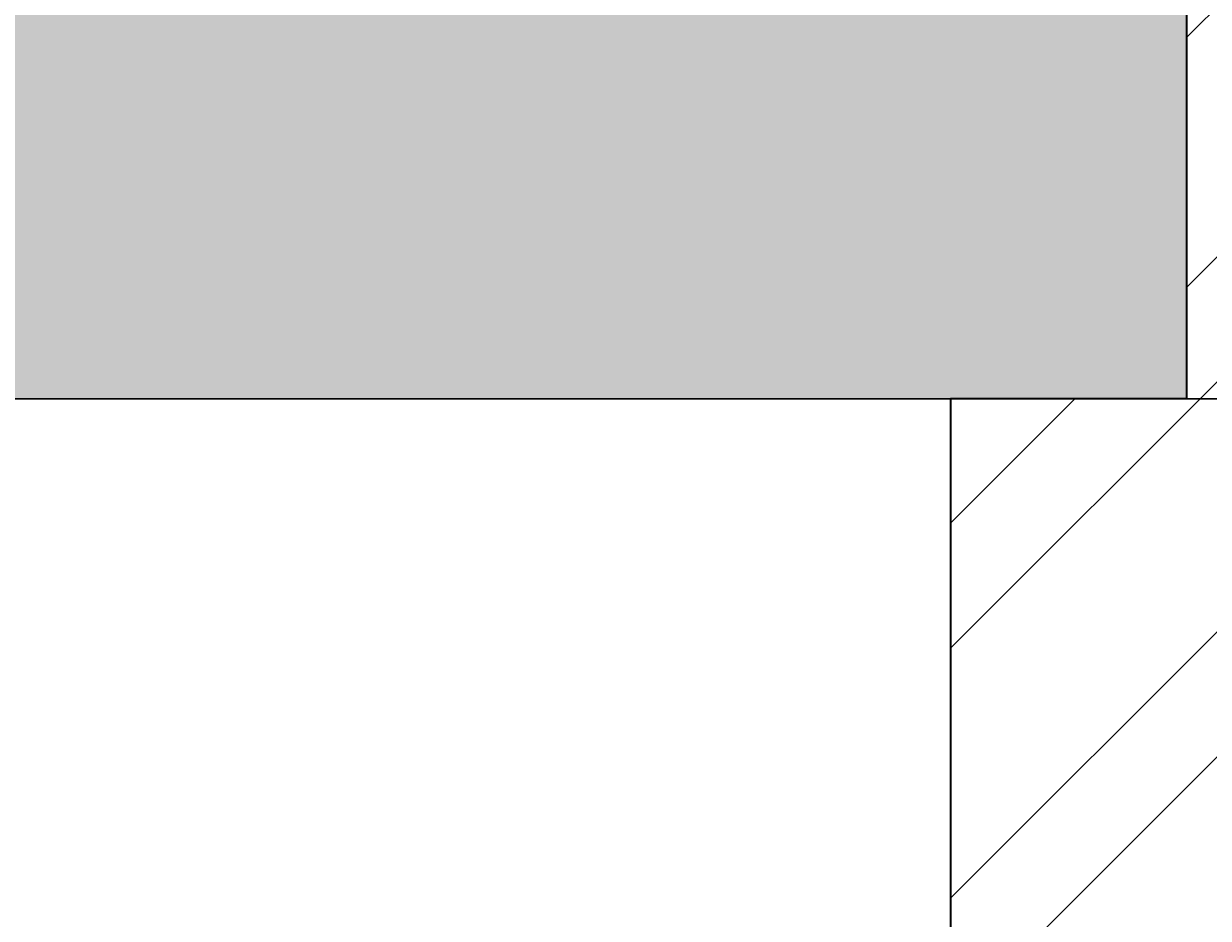
# Model space of a CAD drawing. Units: inches. Extents: x -301 to 715, y -607 to 364.
# Tile 8 of 141: x -66 to -41, y -492 to -474. Entities that reach past the tile are written whole.
import ezdxf

# ---------------------------------------------------------------- set-up
doc = ezdxf.new("R2010")
doc.units = ezdxf.units.IN
doc.header["$MEASUREMENT"] = 0
for name, color, linetype, lineweight in [('A-ANNO-DIMS', 2, 'Continuous', 18), ('A-GRND', 7, 'Continuous', 25), ('A-SECT', 1, 'Continuous', 35), ('A-SECT-PATT', 8, 'Continuous', 13), ('S-FNDN', 2, 'Continuous', 35)]:
    doc.layers.add(name, color=color, linetype=linetype, lineweight=lineweight)
doc.styles.get("Standard").update_dxf_attribs({"font": 'arial.ttf'})
doc.dimstyles.get("Standard").update_dxf_attribs({"dimtxt": 0.18, "dimasz": 0.18, "dimexe": 0.18, "dimexo": 0.0625, "dimgap": 0.09, "dimtad": 0, "dimtih": 1, "dimtoh": 1, "dimdec": 1, "dimzin": 0, "dimdsep": 46, "dimlunit": 4, "dimtxsty": 'Standard', "dimcen": 0.09, "dimclrd": 3, "dimclre": 4, "dimclrt": 6, "dimadec": 0, "dimazin": 0, "dimtfac": 1, "dimtdec": 1, "dimtofl": 0, "dimtmove": 0, "dimatfit": 3, "dimfxl": 1, "dimtfill": 2, "dimtfillclr": 51, "dimtolj": 1, "dimtzin": 0, "dimarcsym": 0})

# ---------------------------------------------------------------- blocks, each defined once
blk = doc.blocks.new('*D179')
at = {"layer": 'A-ANNO-DIMS', "color": 4, "lineweight": -2, "transparency": 16777216}
for p, q in [((-87.981, -433.54), (-87.981, -573.809)), ((-35.282, -463.54), (-35.282, -573.809))]:
    blk.add_line(p, q, dxfattribs=at)
at = {"layer": 'A-ANNO-DIMS', "color": 3, "lineweight": -2, "transparency": 16777216}
for p, q in [((-87.801, -573.629), (-62.174, -573.629)), ((-35.462, -573.629), (-61.089, -573.629))]:
    blk.add_line(p, q, dxfattribs=at)
at = {"layer": 'A-ANNO-DIMS', "color": 3, "transparency": 16777216}
for points in [[(-87.801, -573.599), (-87.801, -573.659), (-87.981, -573.629)], [(-35.462, -573.599), (-35.462, -573.659), (-35.282, -573.629)]]:
    blk.add_solid(points, dxfattribs=at)
at = {"layer": 'Defpoints', "color": 0, "transparency": 16777216}
for p in [(-87.981, -433.477), (-35.282, -463.477), (-35.282, -573.629)]:
    blk.add_point(p, dxfattribs=at)
at = {"layer": 'A-ANNO-DIMS', "color": 6, "transparency": 16777216, "insert": (-61.631, -573.629), "char_height": 0.18, "attachment_point": 5, "bg_fill": 1, "box_fill_scale": 1.25, "bg_fill_color": 51, "bg_fill_transparency": 0}
blk.add_mtext('\\A1;4\'-4 1/2"', dxfattribs=at)
blk = doc.blocks.new('*D190')
at = {"layer": 'A-ANNO-DIMS', "color": 4, "lineweight": -2, "transparency": 16777216}
for p, q in [((129.193, -481.477), (-266.112, -481.477)), ((124.193, -511.477), (-266.112, -511.477))]:
    blk.add_line(p, q, dxfattribs=at)
at = {"layer": 'A-ANNO-DIMS', "color": 3, "lineweight": -2, "transparency": 16777216}
for p, q in [((-265.932, -481.657), (-265.932, -496.296)), ((-265.932, -511.297), (-265.932, -496.659))]:
    blk.add_line(p, q, dxfattribs=at)
at = {"layer": 'A-ANNO-DIMS', "color": 3, "transparency": 16777216}
for points in [[(-265.962, -481.657), (-265.902, -481.657), (-265.932, -481.477)], [(-265.962, -511.297), (-265.902, -511.297), (-265.932, -511.477)]]:
    blk.add_solid(points, dxfattribs=at)
at = {"layer": 'Defpoints', "color": 0, "transparency": 16777216}
for p in [(129.255, -481.477), (-265.932, -511.477), (124.255, -511.477)]:
    blk.add_point(p, dxfattribs=at)
at = {"layer": 'A-ANNO-DIMS', "color": 6, "transparency": 16777216, "insert": (-265.932, -496.477), "char_height": 0.18, "attachment_point": 5, "bg_fill": 1, "box_fill_scale": 1.25, "bg_fill_color": 51, "bg_fill_transparency": 0}
blk.add_mtext('\\A1;2\'-6"', dxfattribs=at)
blk = doc.blocks.new('*D191')
at = {"layer": 'A-ANNO-DIMS', "color": 4, "lineweight": -2, "transparency": 16777216}
for p, q in [((129.193, -481.477), (-266.112, -481.477)), ((114.193, -540.477), (-266.112, -540.477))]:
    blk.add_line(p, q, dxfattribs=at)
at = {"layer": 'A-ANNO-DIMS', "color": 3, "lineweight": -2, "transparency": 16777216}
for p, q in [((-265.932, -481.657), (-265.932, -510.797)), ((-265.932, -540.297), (-265.932, -511.158))]:
    blk.add_line(p, q, dxfattribs=at)
at = {"layer": 'A-ANNO-DIMS', "color": 3, "transparency": 16777216}
for points in [[(-265.962, -481.657), (-265.902, -481.657), (-265.932, -481.477)], [(-265.962, -540.297), (-265.902, -540.297), (-265.932, -540.477)]]:
    blk.add_solid(points, dxfattribs=at)
at = {"layer": 'Defpoints', "color": 0, "transparency": 16777216}
for p in [(129.255, -481.477), (-265.932, -540.477), (114.255, -540.477)]:
    blk.add_point(p, dxfattribs=at)
at = {"layer": 'A-ANNO-DIMS', "color": 6, "transparency": 16777216, "insert": (-265.932, -510.977), "char_height": 0.18, "attachment_point": 5, "bg_fill": 1, "box_fill_scale": 1.25, "bg_fill_color": 51, "bg_fill_transparency": 0}
blk.add_mtext('\\A1;4\'-11"', dxfattribs=at)

msp = doc.modelspace()

# ---------------------------------------------------------------- hatches: boundary and pattern name
at = {"layer": 'A-SECT-PATT'}
h = msp.add_hatch(dxfattribs=at)
h.set_pattern_fill('ANSI32', color=256, scale=15)
h.set_pattern_definition([(45, (10.321, 33.8764), (-3.977476, 3.977476), []), (45, (12.973, 33.8764), (-3.977476, 3.977476), [])])
h.paths.add_polyline_path([(-185.282, -324.477), (-199.282, -324.477), (-199.282, -329.477), (-194.282, -329.477), (-194.282, -353.477), (-185.282, -353.477)])
h.paths.add_polyline_path([(-185.282, -361.477), (-193.904, -361.477), (-193.982, -377.537), (-185.282, -377.537)])
h.paths.add_polyline_path([(143.218, -329.477), (148.218, -329.477), (148.218, -324.477), (134.255, -324.477), (134.255, -353.477), (143.218, -353.477)])
h.paths.add_polyline_path([(143.218, -361.477), (134.255, -361.477), (134.255, -377.477), (143.218, -377.477)])
h.paths.add_polyline_path([(-185.282, -439.477), (-194.282, -439.477), (-194.282, -463.477), (-185.282, -463.477)])
h.paths.add_polyline_path([(-185.282, -471.477), (-194.282, -471.477), (-194.282, -481.477), (-185.282, -481.477)])
h.paths.add_polyline_path([(-185.282, -463.477), (-194.282, -463.477), (-194.282, -466.477), (-185.282, -466.477)])
h.paths.add_polyline_path([(-185.282, -466.477), (-194.282, -466.477), (-194.282, -471.477), (-185.282, -471.477)])
h.paths.add_polyline_path([(-180.282, -481.477), (-185.282, -481.477), (-194.282, -481.477), (-199.282, -481.477), (-199.282, -493.477), (-180.282, -493.477)])
h.paths.add_polyline_path([(-175.282, -493.477), (-180.282, -493.477), (-199.282, -493.477), (-204.282, -493.477), (-204.282, -511.477), (-175.282, -511.477)])
h.paths.add_polyline_path([(-170.282, -511.477), (-175.282, -511.477), (-204.282, -511.477), (-209.282, -511.477), (-209.282, -535.477), (-170.282, -535.477)])
h.paths.add_polyline_path([(-35.282, -463.477), (-41.282, -463.477), (-41.282, -466.477), (-35.282, -466.477)])
h.paths.add_polyline_path([(-35.282, -466.477), (-41.282, -466.477), (-41.282, -471.477), (-35.282, -471.477)])
h.paths.add_polyline_path([(-35.282, -471.477), (-41.282, -471.477), (-41.282, -481.477), (-35.282, -481.477)])
h.paths.add_polyline_path([(-30.282, -481.477), (-46.282, -481.477), (-46.282, -493.477), (-30.282, -493.477)])
h.paths.add_polyline_path([(-25.282, -493.477), (-30.282, -493.477), (-46.282, -493.477), (-51.282, -493.477), (-51.282, -511.477), (-25.282, -511.477)])
h.paths.add_polyline_path([(-20.282, -511.477), (-25.282, -511.477), (-51.282, -511.477), (-56.282, -511.477), (-56.282, -535.477), (-20.282, -535.477)])
h.paths.add_polyline_path([(143.218, -463.477), (134.255, -463.477), (134.255, -466.477), (143.218, -466.477)])
h.paths.add_polyline_path([(143.218, -466.477), (134.255, -466.477), (134.255, -471.477), (143.218, -471.477)])
h.paths.add_polyline_path([(143.218, -471.477), (134.255, -471.477), (134.255, -481.477), (143.218, -481.477)])
h.paths.add_polyline_path([(148.255, -481.477), (143.255, -481.477), (134.255, -481.477), (129.255, -481.477), (129.255, -493.477), (148.255, -493.477)])
h.paths.add_polyline_path([(153.255, -493.477), (148.255, -493.477), (129.255, -493.477), (124.255, -493.477), (124.255, -511.477), (153.255, -511.477)])
h.paths.add_polyline_path([(158.255, -511.477), (153.255, -511.477), (124.255, -511.477), (119.255, -511.477), (119.255, -535.477), (158.255, -535.477)])
h = msp.add_hatch(dxfattribs=at)
h.set_pattern_fill('AR-CONC', color=256, scale=0.5)
h.set_pattern_definition([(50, (10.3213, 33.8764), (3.586301, -0.31376), [0.375, -4.125]), (355, (10.3213, 33.8764), (-0.693757, 3.76096), [0.3, -3.3]), (100.45144, (10.62, 33.8502), (2.892544, 3.4472), [0.3187, -3.50571]), (46.1842, (10.3213, 34.8764), (5.336207, -0.827596), [0.5625, -6.1875]), (96.6356, (10.766, 34.8074), (4.67331, 4.870593), [0.47805, -5.25857]), (351.1842, (10.321, 34.8764), (4.67331, 4.870593), [0.45, -4.95]), (21, (10.8213, 34.6264), (2.984535, -2.013094), [0.375, -4.125]), (326, (10.8213, 34.6264), (1.216577, 3.62575), [0.3, -3.3]), (71.45144, (11.07, 34.4586), (4.201112, 1.612656), [0.3187, -3.50571]), (37.5, (10.3213, 33.8764), (0.0607993, 1.6644693), [0, -3.26, 0, -3.35, 0, -3.3125]), (7.5, (10.3213, 33.8764), (1.3153477, 1.9720586), [0, -1.91, 0, -3.185, 0, -1.2625]), (327.5, (9.2063, 33.8764), (2.6691122, -0.1127744), [0, -1.25, 0, -3.9, 0, -5.175]), (317.5, (8.7063, 33.8764), (2.915931, 0.500525), [0, -1.625, 0, -2.59, 0, -3.675])])
h.paths.add_polyline_path([(-56.282, -535.477), (-61.282, -535.477), (-61.282, -540.477), (-15.282, -540.477), (-15.282, -535.477), (-20.282, -535.477)])
h.paths.add_polyline_path([(119.255, -535.477), (114.255, -535.477), (114.255, -540.477), (163.255, -540.477), (163.255, -535.477), (158.255, -535.477)])
h.paths.add_polyline_path([(-206.282, -471.477), (-209.282, -471.477), (-209.282, -481.477), (-206.282, -481.477), (-194.282, -481.477), (-194.282, -471.477)])
h.paths.add_polyline_path([(-41.282, -481.477), (-41.282, -471.477), (-185.282, -471.477), (-185.282, -481.477), (-180.282, -481.477)])
h.paths.add_polyline_path([(134.255, -481.477), (134.255, -471.477), (-35.282, -471.477), (-35.282, -481.477), (-30.282, -481.477)])
h.paths.add_polyline_path([(155.218, -481.477), (158.218, -481.477), (158.218, -471.477), (153.218, -471.477), (143.218, -471.477), (143.218, -481.477), (148.255, -481.477)])
h.paths.add_polyline_path([(-193.88, -356.477), (-193.904, -361.477), (143.218, -361.477), (143.218, -356.477)])

# ---------------------------------------------------------------- linework, layer by layer
at = {"layer": 'A-GRND'}
msp.add_line((-206.282, -481.477), (155.218, -481.477), dxfattribs=at)
at = {"layer": 'A-SECT'}
msp.add_line((-41.282, -361.477), (-41.282, -481.477), dxfattribs=at)
at = {"layer": 'S-FNDN'}
for p, q in [((-41.282, -481.477), (-46.282, -481.477)), ((-46.282, -481.477), (-46.282, -493.477))]:
    msp.add_line(p, q, dxfattribs=at)

# ---------------------------------------------------------------- dimensions: what is measured, and where the dimension line sits
at = {"layer": 'A-ANNO-DIMS'}
dim = msp.add_linear_dim(base=(-35.282, -573.629), p1=(-87.981, -433.477), p2=(-35.282, -463.477), dimstyle='Standard', override={"dimdec": 1, "dimlfac": 1, "dimrnd": 0, "dimzin": 1, "dimdsep": 46, "dimlunit": 4, "dimfrac": 2}, dxfattribs=at)
dim.commit()
dim.dimension.update_dxf_attribs({"geometry": '*D179', "text_midpoint": (-61.631, -573.629)})
for base, p2, picture, middle in [((-265.932, -540.477), (114.255, -540.477), '*D191', (-265.932, -510.977)), ((-265.932, -511.477), (124.255, -511.477), '*D190', (-265.932, -496.477))]:
    dim = msp.add_linear_dim(base=base, p1=(129.255, -481.477), p2=p2, angle=90, dimstyle='Standard', override={"dimdec": 1, "dimlfac": 1, "dimrnd": 0, "dimzin": 1, "dimdsep": 46, "dimlunit": 4, "dimfrac": 2}, dxfattribs=at)
    dim.commit()
    dim.dimension.update_dxf_attribs({"geometry": picture, "text_midpoint": middle})

doc.saveas('drawing.dxf')
